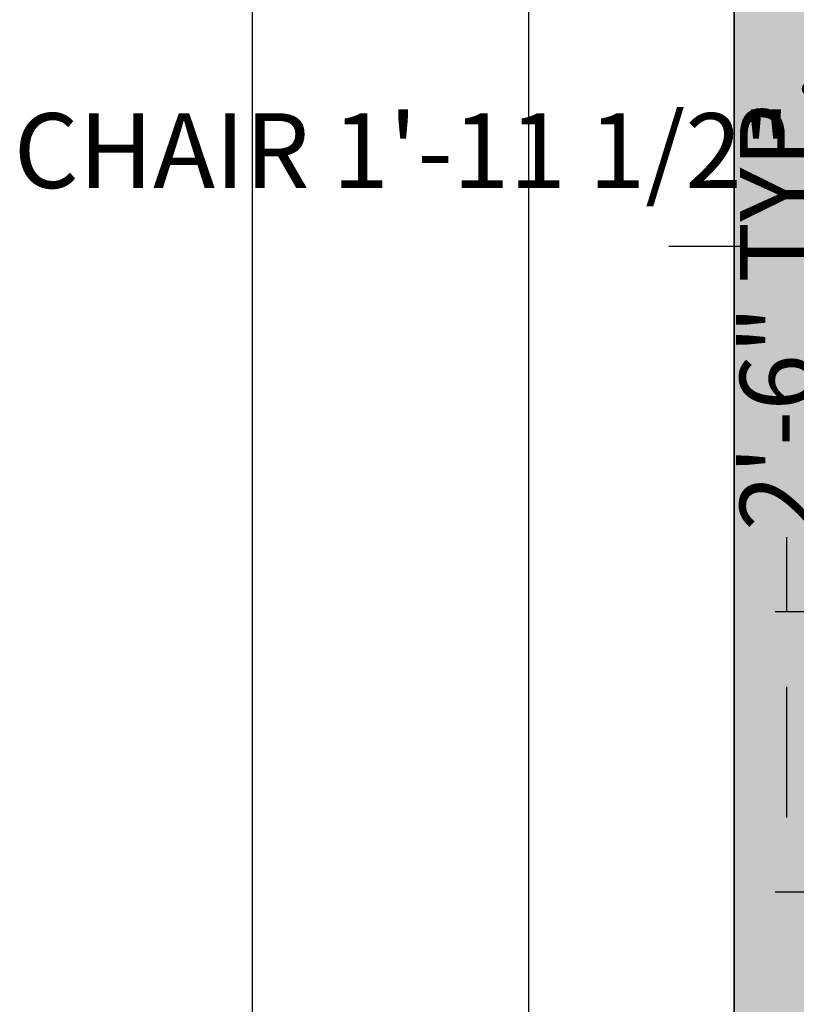
# Model space of a CAD drawing. Units: inches. Extents: x 2408 to 5087, y 2429 to 5085.
# Tile 2 of 12: x 2408 to 2491, y 2570 to 2676. Entities that reach past the tile are written whole.
import ezdxf

# ---------------------------------------------------------------- set-up
doc = ezdxf.new("R2010")
doc.units = ezdxf.units.IN
for name, color, linetype, lineweight in [('A-ANNO-DIMS', 2, 'Continuous', 18), ('A-WALL', 7, 'Continuous', 35), ('A-WALL-PATT', 252, 'Continuous', 13)]:
    doc.layers.add(name, color=color, linetype=linetype, lineweight=lineweight)
doc.styles.get("Standard").update_dxf_attribs({"font": 'arial.ttf'})
doc.dimstyles.new('ISO-25', dxfattribs={"dimtxt": 8, "dimasz": 8, "dimexe": 1.25, "dimexo": 0.625, "dimtad": 0, "dimdec": 1, "dimlunit": 4, "dimtxsty": 'Standard', "dimcen": 2.5, "dimadec": 0, "dimazin": 0, "dimtfac": 1, "dimtdec": 1, "dimtmove": 0, "dimatfit": 3, "dimfxl": 1, "dimarcsym": 0})

# ---------------------------------------------------------------- blocks, each defined once
blk = doc.blocks.new('*D2')
at = {"layer": 'A-ANNO-DIMS', "color": 0, "lineweight": -2, "transparency": 16777216}
for p, q in [((2483.87, 3017.05), (2461.26, 3017.05)), ((2462.51, 3009.05), (2462.51, 2772.63)), ((2462.51, 2521.05), (2462.51, 2757.48)), ((2483.87, 2513.05), (2461.26, 2513.05))]:
    blk.add_line(p, q, dxfattribs=at)
at = {"layer": 'A-ANNO-DIMS', "color": 0, "transparency": 16777216}
for points in [[(2461.17, 3009.05), (2463.84, 3009.05), (2462.51, 3017.05)], [(2461.17, 2521.05), (2463.84, 2521.05), (2462.51, 2513.05)]]:
    blk.add_solid(points, dxfattribs=at)
at = {"layer": 'Defpoints', "color": 0, "transparency": 16777216}
for p in [(2484.49, 3017.05), (2462.51, 2513.05), (2484.49, 2513.05)]:
    blk.add_point(p, dxfattribs=at)
at = {"layer": 'A-ANNO-DIMS', "color": 0, "transparency": 16777216, "insert": (2462.51, 2765.05), "char_height": 8, "attachment_point": 5, "rotation": 90}
blk.add_mtext("42'", dxfattribs=at)
blk = doc.blocks.new('*D30')
at = {"layer": 'A-ANNO-DIMS', "color": 0, "lineweight": -2, "transparency": 16777216}
for p, q in [((2490.13, 2612.41), (2490.13, 2620.41)), ((2494, 2612.41), (2488.88, 2612.41)), ((2490.13, 2590.43), (2490.13, 2604.41)), ((2494, 2582.43), (2488.88, 2582.43))]:
    blk.add_line(p, q, dxfattribs=at)
at = {"layer": 'A-ANNO-DIMS', "color": 0, "transparency": 16777216}
for points in [[(2488.79, 2604.41), (2491.46, 2604.41), (2490.13, 2612.41)], [(2488.79, 2590.43), (2491.46, 2590.43), (2490.13, 2582.43)]]:
    blk.add_solid(points, dxfattribs=at)
at = {"layer": 'Defpoints', "color": 0, "transparency": 16777216}
for p in [(2490.13, 2612.41), (2494.62, 2612.41), (2494.62, 2582.43)]:
    blk.add_point(p, dxfattribs=at)
at = {"layer": 'A-ANNO-DIMS', "color": 0, "transparency": 16777216, "insert": (2490.13, 2645.49), "char_height": 8, "attachment_point": 5, "rotation": 90}
blk.add_mtext('2\'-6" TYP.', dxfattribs=at)
blk = doc.blocks.new('*D45')
at = {"layer": 'A-ANNO-DIMS', "color": 0, "lineweight": -2, "transparency": 16777216}
for p, q in [((2525.6, 2657.87), (2525.6, 2661.99)), ((2548.93, 2657.87), (2548.93, 2661.99)), ((2525.6, 2660.74), (2517.6, 2660.74)), ((2540.93, 2660.74), (2533.6, 2660.74))]:
    blk.add_line(p, q, dxfattribs=at)
at = {"layer": 'A-ANNO-DIMS', "color": 0, "transparency": 16777216}
for points in [[(2533.6, 2662.08), (2533.6, 2659.41), (2525.6, 2660.74)], [(2540.93, 2662.08), (2540.93, 2659.41), (2548.93, 2660.74)]]:
    blk.add_solid(points, dxfattribs=at)
at = {"layer": 'Defpoints', "color": 0, "transparency": 16777216}
for p in [(2525.6, 2660.74), (2525.6, 2657.24), (2548.93, 2657.24)]:
    blk.add_point(p, dxfattribs=at)
at = {"layer": 'A-ANNO-DIMS', "color": 0, "transparency": 16777216, "insert": (2461.28, 2660.74), "char_height": 8, "attachment_point": 5}
blk.add_mtext('CHAIR 1\'-11 1/2" TYP.', dxfattribs=at)
blk = doc.blocks.new('*D66')
at = {"layer": 'A-ANNO-DIMS', "color": 0, "lineweight": -2, "transparency": 16777216}
for p, q in [((2483.87, 3017.05), (2431.68, 3017.05)), ((2432.93, 3009.05), (2432.93, 2767.25)), ((2432.93, 2477.75), (2432.93, 2719.56)), ((2461.25, 2469.75), (2431.68, 2469.75))]:
    blk.add_line(p, q, dxfattribs=at)
at = {"layer": 'A-ANNO-DIMS', "color": 0, "transparency": 16777216}
for points in [[(2431.59, 3009.05), (2434.26, 3009.05), (2432.93, 3017.05)], [(2431.59, 2477.75), (2434.26, 2477.75), (2432.93, 2469.75)]]:
    blk.add_solid(points, dxfattribs=at)
at = {"layer": 'Defpoints', "color": 0, "transparency": 16777216}
for p in [(2432.93, 3017.05), (2484.49, 3017.05), (2461.88, 2469.75)]:
    blk.add_point(p, dxfattribs=at)
at = {"layer": 'A-ANNO-DIMS', "color": 0, "transparency": 16777216, "insert": (2432.93, 2743.4), "char_height": 8, "attachment_point": 5, "rotation": 90}
blk.add_mtext('45\'-7 1/2"', dxfattribs=at)
blk = doc.blocks.new('*D74')
at = {"layer": 'A-ANNO-DIMS', "color": 0, "lineweight": -2, "transparency": 16777216}
for p, q in [((2493.49, 2623.18), (2493.49, 2652.75)), ((2523.49, 2623.18), (2523.49, 2652.75)), ((2485.49, 2651.5), (2477.49, 2651.5)), ((2493.49, 2651.5), (2497.17, 2651.5)), ((2523.49, 2651.5), (2519.82, 2651.5)), ((2531.49, 2651.5), (2539.49, 2651.5))]:
    blk.add_line(p, q, dxfattribs=at)
at = {"layer": 'A-ANNO-DIMS', "color": 0, "transparency": 16777216}
for points in [[(2485.49, 2652.84), (2485.49, 2650.17), (2493.49, 2651.5)], [(2531.49, 2652.84), (2531.49, 2650.17), (2523.49, 2651.5)]]:
    blk.add_solid(points, dxfattribs=at)
at = {"layer": 'Defpoints', "color": 0, "transparency": 16777216}
for p in [(2523.49, 2651.5), (2493.49, 2622.55), (2523.49, 2622.55)]:
    blk.add_point(p, dxfattribs=at)
at = {"layer": 'A-ANNO-DIMS', "color": 0, "transparency": 16777216, "insert": (2508.49, 2651.5), "char_height": 8, "attachment_point": 5}
blk.add_mtext('2\'-6"', dxfattribs=at)

msp = doc.modelspace()

# ---------------------------------------------------------------- hatches: boundary and pattern name
at = {"layer": 'A-WALL-PATT'}
h = msp.add_hatch(color=256, dxfattribs=at)
h.dxf.hatch_style = 1
h.paths.add_polyline_path([(2493.49, 2613.55), (2523.49, 2613.55), (2523.49, 2622.55), (2493.49, 2622.55), (2493.49, 2714.8), (2484.49, 2714.8), (2484.49, 2497.75), (2493.49, 2497.75)])
h.paths.add_polyline_path([(2613.49, 2615.42), (2613.49, 2622.55), (2583.49, 2622.55), (2583.49, 2613.55), (2613.46, 2613.55, -0.009707)])
h.paths.add_polyline_path([(2823.49, 2634.55), (2814.49, 2634.55), (2814.49, 2622.55), (2694.49, 2622.55), (2694.49, 2670.55), (2706.49, 2670.55), (2706.49, 2675.05), (2694.49, 2675.05), (2694.49, 2750.05), (2685.49, 2750.05), (2685.49, 2622.55), (2661.49, 2622.55), (2661.49, 2613.55), (2814.49, 2613.55), (2814.49, 2522.05), (2688.49, 2522.05), (2688.49, 2513.05), (2823.49, 2513.05)])
h.paths.add_polyline_path([(2823.49, 2837.05), (2814.49, 2837.05), (2814.49, 2819.05), (2685.49, 2819.05), (2685.49, 2786.05), (2694.49, 2786.05), (2694.49, 2810.05), (2814.49, 2810.05), (2814.49, 2772.55), (2823.49, 2772.55)])
h.paths.add_polyline_path([(2694.49, 2964.55), (2595.49, 2964.55), (2595.49, 3008.05), (2601.49, 3008.05), (2601.49, 3017.05), (2484.49, 3017.05), (2484.49, 2972.05), (2493.49, 2972.05), (2493.49, 3008.05), (2586.49, 3008.05), (2586.49, 2955.55), (2685.49, 2955.55), (2685.49, 2854.87), (2694.49, 2854.87)])
h.paths.add_polyline_path([(2493.49, 2867.05), (2595.49, 2867.05), (2595.49, 2876.05), (2493.49, 2876.05), (2493.49, 2912.05), (2484.49, 2912.05), (2484.49, 2774.8), (2493.49, 2774.8)])
h.paths.add_polyline_path([(2595.49, 2814.55), (2493.49, 2814.55), (2493.49, 2810.05), (2595.49, 2810.05)], flags=17)
h.paths.add_polyline_path([(2724.49, 3017.05), (2625.49, 3017.05), (2625.49, 3008.05), (2685.49, 3008.05), (2685.49, 2994.55), (2694.49, 2994.55), (2694.49, 3008.05), (2724.49, 3008.05)])
h.paths.add_polyline_path([(2823.49, 3017.05), (2784.49, 3017.05), (2784.49, 3008.05), (2814.49, 3008.05), (2814.49, 2913.55), (2814.56, 2897.05), (2823.49, 2897.05)])
h.paths.add_polyline_path([(2823.49, 2712.55), (2814.61, 2712.55), (2814.66, 2701.27), (2814.49, 2701.27), (2814.49, 2675.05), (2740.99, 2675.05), (2740.99, 2687.05), (2736.49, 2687.05), (2736.49, 2670.55), (2814.49, 2670.55), (2814.49, 2658.55), (2823.49, 2658.55)], flags=17)

# ---------------------------------------------------------------- linework, layer by layer
at = {"layer": 'A-WALL'}
msp.add_line((2484.49, 3017.05), (2484.49, 2497.75), dxfattribs=at)

# ---------------------------------------------------------------- dimensions: what is measured, and where the dimension line sits
at = {"layer": 'A-ANNO-DIMS'}
for base, p1, p2, override, picture, middle in [((2432.93, 3017.05), (2461.88, 2469.75), (2484.49, 3017.05), {"dimdec": 1, "dimlfac": 1, "dimrnd": 0, "dimzin": 1, "dimdsep": 46, "dimlunit": 4, "dimfrac": 2}, '*D66', (2432.93, 2743.4)), ((2462.51, 2513.05), (2484.49, 3017.05), (2484.49, 2513.05), {"dimclrd": 0, "dimclre": 0, "dimclrt": 0}, '*D2', (2462.51, 2765.05))]:
    dim = msp.add_linear_dim(base=base, p1=p1, p2=p2, angle=90, dimstyle='ISO-25', override=override, dxfattribs=at)
    dim.commit()
    dim.dimension.update_dxf_attribs({"geometry": picture, "text_midpoint": middle})
for base, p1, p2, angle, text, picture, middle in [((2525.6, 2660.74), (2548.93, 2657.24), (2525.6, 2657.24), 180, 'CHAIR <> TYP.', '*D45', (2461.28, 2660.74)), ((2490.13, 2612.41), (2494.62, 2582.43), (2494.62, 2612.41), 90, '<> TYP.', '*D30', (2490.13, 2645.49))]:
    dim = msp.add_linear_dim(base=base, p1=p1, p2=p2, angle=angle, text=text, dimstyle='ISO-25', override={"dimdec": 1, "dimlfac": 1, "dimrnd": 0, "dimzin": 1, "dimdsep": 46, "dimlunit": 4, "dimfrac": 2}, dxfattribs=at)
    dim.commit()
    dim.dimension.update_dxf_attribs({"geometry": picture, "text_midpoint": middle})
dim = msp.add_linear_dim(base=(2523.49, 2651.5), p1=(2493.49, 2622.55), p2=(2523.49, 2622.55), dimstyle='ISO-25', override={"dimdec": 1, "dimlfac": 1, "dimrnd": 0, "dimzin": 1, "dimdsep": 46, "dimlunit": 4, "dimfrac": 2}, dxfattribs=at)
dim.commit()
dim.dimension.update_dxf_attribs({"geometry": '*D74', "text_midpoint": (2508.49, 2651.5)})

doc.saveas('drawing.dxf')
